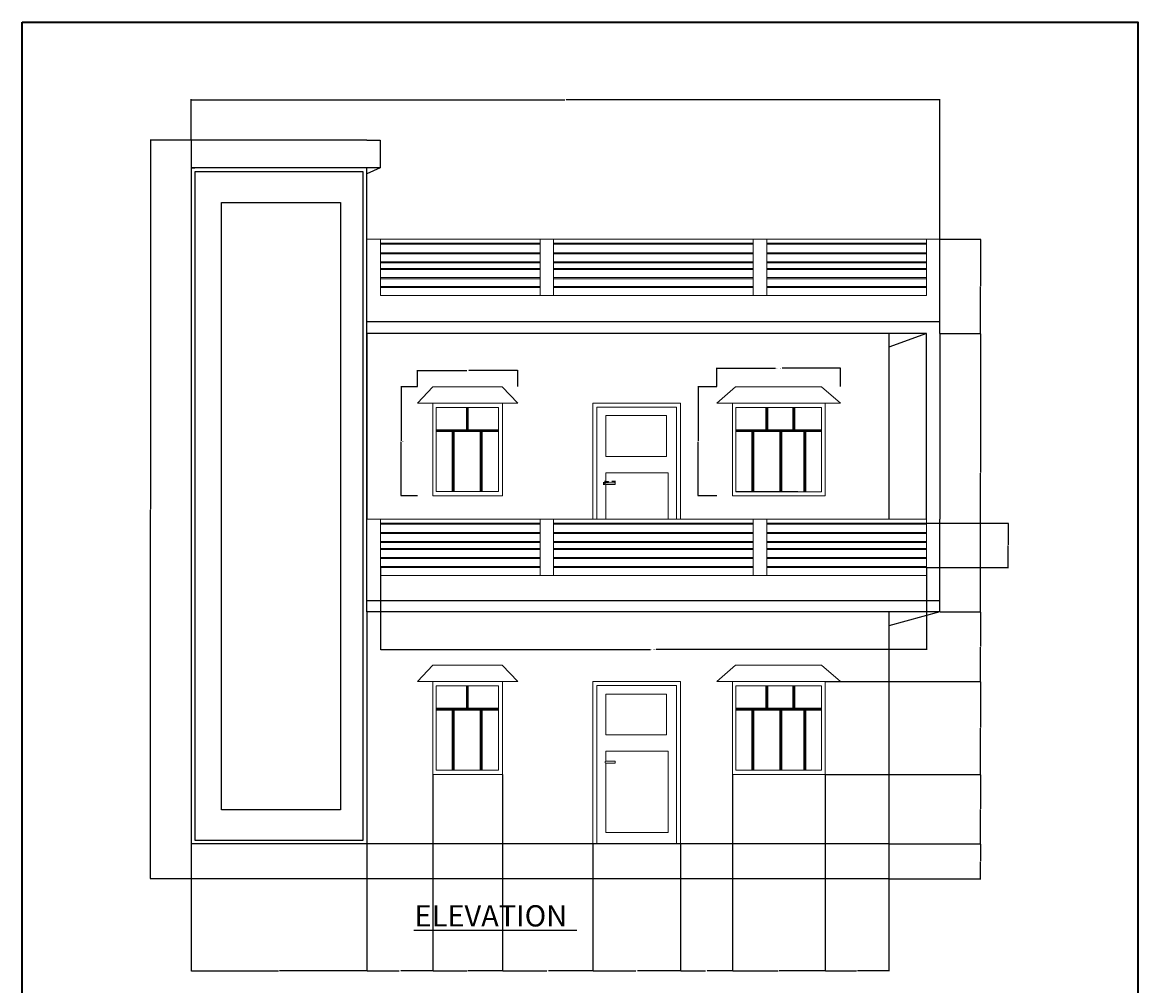
# Model space of a CAD drawing. Units: inches. Extents: x 1623 to 2200, y 2019 to 3010.
# Tile 6 of 6: x 1623 to 2200, y 2512 to 3010. Entities that reach past the tile are written whole.
import ezdxf

# ---------------------------------------------------------------- set-up
doc = ezdxf.new("R2010")
doc.units = ezdxf.units.IN
for name, color, linetype, lineweight in [('A-ANNO-DIMS', 2, 'Continuous', 18), ('A-ANNO-TITL', 7, 'Continuous', 25), ('A-ANNO-TTLB', 7, 'Continuous', 35), ('A-ELEV', 7, 'Continuous', 25), ('A-ELEV-DOOR', 3, 'Continuous', 18), ('A-ELEV-GLAZ', 4, 'Continuous', 18), ('A-ELEV-RAIL', 7, 'Continuous', 18)]:
    doc.layers.add(name, color=color, linetype=linetype, lineweight=lineweight)
doc.styles.get("Standard").update_dxf_attribs({"font": 'arial.ttf'})
doc.dimstyles.get("Standard").update_dxf_attribs({"dimtxt": 0.18, "dimasz": 0.18, "dimexe": 0.18, "dimexo": 0.0625, "dimgap": 0.09, "dimtad": 0, "dimtih": 1, "dimtoh": 1, "dimdec": 4, "dimzin": 0, "dimdsep": 46, "dimtxsty": 'Standard', "dimcen": 0.09, "dimadec": 0, "dimazin": 0, "dimtfac": 1, "dimtdec": 4, "dimtofl": 0, "dimtmove": 0, "dimatfit": 3, "dimfxl": 1, "dimtolj": 1, "dimtzin": 0, "dimarcsym": 0})

# ---------------------------------------------------------------- blocks, each defined once
blk = doc.blocks.new('WIN-HOODED-36-ELEV')
for p, q in [((0, 48), (8, 56.49)), ((8, 56.49), (43.77, 56.49)), ((52, 48), (43.77, 56.49)), ((8, 48), (0, 48)), ((8, 48), (8, 0)), ((44, 48), (8, 48)), ((44, 48), (44, 0)), ((44, 48), (52, 48)), ((25.79, 45.8), (25.29, 45.8)), ((25.29, 45.8), (25.29, 34.28)), ((25.79, 45.8), (25.79, 34.28)), ((26.29, 45.8), (25.79, 45.8)), ((26.29, 34.28), (26.29, 45.8)), ((9.7, 34.28), (41.87, 34.28)), ((9.7, 33.28), (9.7, 33.78)), ((9.7, 33.78), (41.87, 33.78)), ((41.87, 33.28), (9.7, 33.28)), ((18.52, 33.28), (18.02, 33.28)), ((18.02, 33.28), (18.02, 2.25)), ((18.52, 33.28), (18.52, 2.25)), ((19.02, 33.28), (18.52, 33.28)), ((19.02, 2.25), (19.02, 33.28)), ((25.79, 34.28), (26.29, 34.28)), ((32.47, 33.28), (32.47, 2.25)), ((32.97, 33.28), (32.97, 2.25)), ((33.47, 2.25), (33.47, 33.28)), ((41.87, 34.28), (41.87, 33.28)), ((44, 0), (8, 0)), ((18.52, 2.25), (19.02, 2.25))]:
    blk.add_line(p, q)
for points in [[(8, 48), (44, 48), (44, 0), (8, 0)], [(9.7, 45.8), (41.87, 45.8), (41.87, 2.25), (9.7, 2.25)]]:
    blk.add_lwpolyline(points, close=True)
blk = doc.blocks.new('WIN-HOODED-48-ELEV')
for p, q in [((0, 48), (9.64, 56.49)), ((9.64, 56.49), (54.05, 56.49)), ((64, 48), (54.05, 56.49)), ((8, 48), (0, 48)), ((56, 48), (8, 48)), ((8, 48), (8, 0)), ((56, 48), (56, 0)), ((56, 48), (64, 48)), ((25.38, 45.8), (25.38, 34.28)), ((25.88, 45.8), (25.88, 34.28)), ((26.38, 34.28), (26.38, 45.8)), ((39.3, 45.8), (39.3, 34.28)), ((39.8, 45.8), (39.8, 34.28)), ((40.3, 34.28), (40.3, 45.8)), ((9.79, 34.28), (54.04, 34.28)), ((9.79, 33.78), (54.04, 33.78)), ((54.04, 33.28), (9.79, 33.28)), ((18.61, 33.28), (18.11, 33.28)), ((18.11, 33.28), (18.11, 2.25)), ((18.61, 33.28), (18.61, 2.25)), ((19.11, 33.28), (18.61, 33.28)), ((19.11, 2.25), (19.11, 33.28)), ((25.88, 34.28), (26.38, 34.28)), ((32.57, 33.28), (32.57, 2.25)), ((33.07, 33.28), (33.07, 2.25)), ((33.57, 2.25), (33.57, 33.28)), ((45.02, 33.28), (45.02, 2.25)), ((45.52, 33.28), (45.52, 2.25)), ((46.02, 2.25), (46.02, 33.28)), ((56, 0), (8, 0))]:
    blk.add_line(p, q)
blk.add_lwpolyline([(41.96, 2.25), (9.79, 2.25), (9.79, 45.8), (41.96, 45.8)])
blk.add_lwpolyline([(9.79, 45.8), (54.04, 45.8), (54.04, 2.19), (9.79, 2.19)], close=True)
blk = doc.blocks.new('GUARD-INFILL-THREE-BAY')
for p, q in [((0, 22.98), (82.54, 22.98)), ((0, 22.44), (82.54, 22.44)), ((0, 18.02), (82.54, 18.02)), ((0, 17.48), (82.54, 17.48)), ((89.54, 22.98), (192.77, 22.98)), ((89.54, 22.44), (192.77, 22.44)), ((89.54, 18.02), (192.77, 18.02)), ((89.54, 17.48), (192.77, 17.48)), ((199.77, 22.98), (282.36, 22.98)), ((199.77, 22.44), (282.36, 22.44)), ((199.77, 18.02), (282.36, 18.02)), ((199.77, 17.48), (282.36, 17.48)), ((0, 13.4), (82.54, 13.4)), ((0, 12.86), (82.54, 12.86)), ((89.54, 13.4), (192.77, 13.4)), ((89.54, 12.86), (192.77, 12.86)), ((199.77, 13.4), (282.36, 13.4)), ((199.77, 12.86), (282.36, 12.86)), ((0, 9.89), (82.54, 9.89)), ((0, 9.34), (82.54, 9.34)), ((89.54, 9.89), (192.77, 9.89)), ((89.54, 9.34), (192.77, 9.34)), ((199.77, 9.89), (282.36, 9.89)), ((199.77, 9.34), (282.36, 9.34)), ((0, 5.16), (82.54, 5.16)), ((0, 4.62), (82.54, 4.62)), ((0, 0.54), (82.54, 0.54)), ((0, 0), (82.54, 0)), ((89.54, 5.16), (192.77, 5.16)), ((89.54, 4.62), (192.77, 4.62)), ((89.54, 0.54), (192.77, 0.54)), ((89.54, 0), (192.77, 0)), ((199.77, 5.16), (282.36, 5.16)), ((199.77, 4.62), (282.36, 4.62)), ((199.77, 0.54), (282.36, 0.54)), ((199.77, 0), (282.36, 0))]:
    blk.add_line(p, q)
blk = doc.blocks.new('DOOR-LEVER-ELEV')
blk.add_lwpolyline([(0.34, 0.92), (5.29, 0.92), (5.29, 0), (0.34, 0)])
blk.add_arc((0.48, 0.46), 0.478, 106.81153, 253.18847)
blk = doc.blocks.new('*D20')
at = {"layer": 'A-ANNO-DIMS', "color": 0, "lineweight": -2, "transparency": 16777216}
for p, q in [((1827.39, 2822.01), (1818.8, 2822.01)), ((1818.98, 2821.83), (1818.98, 2793.95)), ((1818.98, 2765.7), (1818.98, 2793.58)), ((1827.39, 2765.52), (1818.8, 2765.52))]:
    blk.add_line(p, q, dxfattribs=at)
at = {"layer": 'A-ANNO-DIMS', "color": 0, "transparency": 16777216}
for points in [[(1818.95, 2821.83), (1819.01, 2821.83), (1818.98, 2822.01)], [(1818.95, 2765.7), (1819.01, 2765.7), (1818.98, 2765.52)]]:
    blk.add_solid(points, dxfattribs=at)
at = {"layer": 'Defpoints', "color": 0, "transparency": 16777216}
for p in [(1818.98, 2822.01), (1827.45, 2822.01), (1827.45, 2765.52)]:
    blk.add_point(p, dxfattribs=at)
at = {"layer": 'A-ANNO-DIMS', "color": 0, "transparency": 16777216, "insert": (1818.98, 2793.77), "char_height": 0.18, "attachment_point": 5}
blk.add_mtext('\\A1;HOODED WINDOW 56 TYP.', dxfattribs=at)
blk = doc.blocks.new('*D21')
at = {"layer": 'A-ANNO-DIMS', "color": 0, "lineweight": -2, "transparency": 16777216}
for p, q in [((1827.45, 2822.07), (1827.45, 2830.66)), ((1827.63, 2830.48), (1852.93, 2830.48)), ((1879.27, 2830.48), (1853.98, 2830.48)), ((1879.45, 2822.07), (1879.45, 2830.66))]:
    blk.add_line(p, q, dxfattribs=at)
at = {"layer": 'A-ANNO-DIMS', "color": 0, "transparency": 16777216}
for points in [[(1827.63, 2830.51), (1827.63, 2830.45), (1827.45, 2830.48)], [(1879.27, 2830.51), (1879.27, 2830.45), (1879.45, 2830.48)]]:
    blk.add_solid(points, dxfattribs=at)
at = {"layer": 'Defpoints', "color": 0, "transparency": 16777216}
for p in [(1879.45, 2830.48), (1827.45, 2822.01), (1879.45, 2822.01)]:
    blk.add_point(p, dxfattribs=at)
at = {"layer": 'A-ANNO-DIMS', "color": 0, "transparency": 16777216, "insert": (1853.45, 2830.48), "char_height": 0.18, "attachment_point": 5}
blk.add_mtext('\\A1;52 TYP.', dxfattribs=at)
blk = doc.blocks.new('*D22')
at = {"layer": 'A-ANNO-DIMS', "color": 0, "lineweight": -2, "transparency": 16777216}
for p, q in [((1982.33, 2822.07), (1982.33, 2831.79)), ((1982.51, 2831.61), (2012.63, 2831.61)), ((2046.15, 2831.61), (2016.02, 2831.61)), ((2046.33, 2822.07), (2046.33, 2831.79))]:
    blk.add_line(p, q, dxfattribs=at)
at = {"layer": 'A-ANNO-DIMS', "color": 0, "transparency": 16777216}
for points in [[(1982.51, 2831.64), (1982.51, 2831.58), (1982.33, 2831.61)], [(2046.15, 2831.64), (2046.15, 2831.58), (2046.33, 2831.61)]]:
    blk.add_solid(points, dxfattribs=at)
at = {"layer": 'Defpoints', "color": 0, "transparency": 16777216}
for p in [(2046.33, 2831.61), (1982.33, 2822.01), (2046.33, 2822.01)]:
    blk.add_point(p, dxfattribs=at)
at = {"layer": 'A-ANNO-DIMS', "color": 0, "transparency": 16777216, "insert": (2014.33, 2831.61), "char_height": 0.18, "attachment_point": 5}
blk.add_mtext('\\A1;HOODED WINDOW 64 TYP.', dxfattribs=at)
blk = doc.blocks.new('*D23')
at = {"layer": 'A-ANNO-DIMS', "color": 0, "lineweight": -2, "transparency": 16777216}
for p, q in [((1982.26, 2822.01), (1972.55, 2822.01)), ((1972.73, 2821.83), (1972.73, 2793.95)), ((1972.73, 2765.7), (1972.73, 2793.58)), ((1982.26, 2765.52), (1972.55, 2765.52))]:
    blk.add_line(p, q, dxfattribs=at)
at = {"layer": 'A-ANNO-DIMS', "color": 0, "transparency": 16777216}
for points in [[(1972.7, 2821.83), (1972.76, 2821.83), (1972.73, 2822.01)], [(1972.7, 2765.7), (1972.76, 2765.7), (1972.73, 2765.52)]]:
    blk.add_solid(points, dxfattribs=at)
at = {"layer": 'Defpoints', "color": 0, "transparency": 16777216}
for p in [(1972.73, 2822.01), (1982.33, 2822.01), (1982.33, 2765.52)]:
    blk.add_point(p, dxfattribs=at)
at = {"layer": 'A-ANNO-DIMS', "color": 0, "transparency": 16777216, "insert": (1972.73, 2793.77), "char_height": 0.18, "attachment_point": 5}
blk.add_mtext('\\A1;56 TYP.', dxfattribs=at)
blk = doc.blocks.new('*D24')
at = {"layer": 'A-ANNO-DIMS', "color": 0, "lineweight": -2, "transparency": 16777216}
for p, q in [((1808.33, 2728.48), (1808.33, 2686.01)), ((2090.69, 2728.48), (2090.69, 2686.01)), ((1808.51, 2686.19), (1948.01, 2686.19)), ((2090.51, 2686.19), (1951, 2686.19))]:
    blk.add_line(p, q, dxfattribs=at)
at = {"layer": 'A-ANNO-DIMS', "color": 0, "transparency": 16777216}
for points in [[(1808.51, 2686.22), (1808.51, 2686.16), (1808.33, 2686.19)], [(2090.51, 2686.22), (2090.51, 2686.16), (2090.69, 2686.19)]]:
    blk.add_solid(points, dxfattribs=at)
at = {"layer": 'Defpoints', "color": 0, "transparency": 16777216}
for p in [(1808.33, 2728.54), (2090.69, 2728.54), (2090.69, 2686.19)]:
    blk.add_point(p, dxfattribs=at)
at = {"layer": 'A-ANNO-DIMS', "color": 0, "transparency": 16777216, "insert": (1949.51, 2686.19), "char_height": 0.18, "attachment_point": 5}
blk.add_mtext('\\A1;GUARD INFILL 282 TYP.', dxfattribs=at)
blk = doc.blocks.new('*D25')
at = {"layer": 'A-ANNO-DIMS', "color": 0, "lineweight": -2, "transparency": 16777216}
for p, q in [((2090.75, 2751.52), (2133.22, 2751.52)), ((2133.04, 2751.34), (2133.04, 2740.21)), ((2133.04, 2728.72), (2133.04, 2739.85)), ((2090.75, 2728.54), (2133.22, 2728.54))]:
    blk.add_line(p, q, dxfattribs=at)
at = {"layer": 'A-ANNO-DIMS', "color": 0, "transparency": 16777216}
for points in [[(2133.01, 2751.34), (2133.07, 2751.34), (2133.04, 2751.52)], [(2133.01, 2728.72), (2133.07, 2728.72), (2133.04, 2728.54)]]:
    blk.add_solid(points, dxfattribs=at)
at = {"layer": 'Defpoints', "color": 0, "transparency": 16777216}
for p in [(2090.69, 2751.52), (2133.04, 2751.52), (2090.69, 2728.54)]:
    blk.add_point(p, dxfattribs=at)
at = {"layer": 'A-ANNO-DIMS', "color": 0, "transparency": 16777216, "insert": (2133.04, 2740.03), "char_height": 0.18, "attachment_point": 5}
blk.add_mtext('\\A1;23 TYP.', dxfattribs=at)
blk = doc.blocks.new('*D26')
at = {"layer": 'A-ANNO-DIMS', "color": 0, "lineweight": -2, "transparency": 16777216}
for p, q in [((1924.49, 2772.35), (1924.49, 2773.26)), ((1924.67, 2773.08), (1926.24, 2773.08)), ((1929.6, 2773.08), (1928.04, 2773.08)), ((1929.78, 2772.35), (1929.78, 2773.26))]:
    blk.add_line(p, q, dxfattribs=at)
at = {"layer": 'A-ANNO-DIMS', "color": 0, "transparency": 16777216}
for points in [[(1924.67, 2773.11), (1924.67, 2773.05), (1924.49, 2773.08)], [(1929.6, 2773.11), (1929.6, 2773.05), (1929.78, 2773.08)]]:
    blk.add_solid(points, dxfattribs=at)
at = {"layer": 'Defpoints', "color": 0, "transparency": 16777216}
for p in [(1924.49, 2772.28), (1929.78, 2773.08), (1929.78, 2772.28)]:
    blk.add_point(p, dxfattribs=at)
at = {"layer": 'A-ANNO-DIMS', "color": 0, "transparency": 16777216, "insert": (1927.14, 2773.08), "char_height": 0.18, "attachment_point": 5}
blk.add_mtext('\\A1;LEVER 5 TYP.', dxfattribs=at)
blk = doc.blocks.new('*D27')
at = {"layer": 'A-ANNO-DIMS', "color": 0, "lineweight": -2, "transparency": 16777216}
for p, q in [((1924.43, 2772.28), (1923.52, 2772.28)), ((1924.43, 2771.37), (1923.52, 2771.37)), ((1923.7, 2772.1), (1923.7, 2772.01)), ((1923.7, 2771.55), (1923.7, 2771.65))]:
    blk.add_line(p, q, dxfattribs=at)
at = {"layer": 'A-ANNO-DIMS', "color": 0, "transparency": 16777216}
for points in [[(1923.67, 2772.1), (1923.73, 2772.1), (1923.7, 2772.28)], [(1923.67, 2771.55), (1923.73, 2771.55), (1923.7, 2771.37)]]:
    blk.add_solid(points, dxfattribs=at)
at = {"layer": 'Defpoints', "color": 0, "transparency": 16777216}
for p in [(1923.7, 2772.28), (1924.49, 2772.28), (1924.49, 2771.37)]:
    blk.add_point(p, dxfattribs=at)
at = {"layer": 'A-ANNO-DIMS', "color": 0, "transparency": 16777216, "insert": (1923.7, 2771.83), "char_height": 0.18, "attachment_point": 5}
blk.add_mtext('\\A1;1 TYP.', dxfattribs=at)
blk = doc.blocks.new('*D44')
at = {"layer": 'A-ANNO-DIMS', "color": 0, "lineweight": -2, "transparency": 16777216}
for p, q in [((1710.33, 2949.6), (1710.33, 2970.66)), ((1710.51, 2970.48), (1903.61, 2970.48)), ((2097.51, 2970.48), (1904.4, 2970.48)), ((2097.69, 2898.32), (2097.69, 2970.66))]:
    blk.add_line(p, q, dxfattribs=at)
at = {"layer": 'A-ANNO-DIMS', "color": 0, "transparency": 16777216}
for points in [[(1710.51, 2970.51), (1710.51, 2970.45), (1710.33, 2970.48)], [(2097.51, 2970.51), (2097.51, 2970.45), (2097.69, 2970.48)]]:
    blk.add_solid(points, dxfattribs=at)
at = {"layer": 'Defpoints', "color": 0, "transparency": 16777216}
for p in [(2097.69, 2970.48), (1710.33, 2949.53), (2097.69, 2898.26)]:
    blk.add_point(p, dxfattribs=at)
at = {"layer": 'A-ANNO-DIMS', "color": 0, "transparency": 16777216, "insert": (1904.01, 2970.48), "char_height": 0.18, "attachment_point": 5}
blk.add_mtext('\\A1;387.4', dxfattribs=at)
blk = doc.blocks.new('*D45')
at = {"layer": 'A-ANNO-DIMS', "color": 0, "lineweight": -2, "transparency": 16777216}
for p, q in [((1710.26, 2949.53), (1689.2, 2949.53)), ((1689.38, 2949.35), (1689.38, 2758.71)), ((1689.38, 2567.7), (1689.38, 2758.34)), ((1710.26, 2567.52), (1689.2, 2567.52))]:
    blk.add_line(p, q, dxfattribs=at)
at = {"layer": 'A-ANNO-DIMS', "color": 0, "transparency": 16777216}
for points in [[(1689.35, 2949.35), (1689.41, 2949.35), (1689.38, 2949.53)], [(1689.35, 2567.7), (1689.41, 2567.7), (1689.38, 2567.52)]]:
    blk.add_solid(points, dxfattribs=at)
at = {"layer": 'Defpoints', "color": 0, "transparency": 16777216}
for p in [(1689.38, 2949.53), (1710.33, 2949.53), (1710.33, 2567.52)]:
    blk.add_point(p, dxfattribs=at)
at = {"layer": 'A-ANNO-DIMS', "color": 0, "transparency": 16777216, "insert": (1689.38, 2758.53), "char_height": 0.18, "attachment_point": 5}
blk.add_mtext('\\A1;382', dxfattribs=at)
blk = doc.blocks.new('*D46')
at = {"layer": 'A-ANNO-DIMS', "color": 0, "lineweight": -2, "transparency": 16777216}
for p, q in [((2071.39, 2585.52), (2118.82, 2585.52)), ((2118.64, 2585.34), (2118.64, 2576.7)), ((2118.64, 2567.7), (2118.64, 2576.34)), ((2071.39, 2567.52), (2118.82, 2567.52))]:
    blk.add_line(p, q, dxfattribs=at)
at = {"layer": 'A-ANNO-DIMS', "color": 0, "transparency": 16777216}
for points in [[(2118.61, 2585.34), (2118.67, 2585.34), (2118.64, 2585.52)], [(2118.61, 2567.7), (2118.67, 2567.7), (2118.64, 2567.52)]]:
    blk.add_solid(points, dxfattribs=at)
at = {"layer": 'Defpoints', "color": 0, "transparency": 16777216}
for p in [(2071.33, 2585.52), (2118.64, 2585.52), (2071.33, 2567.52)]:
    blk.add_point(p, dxfattribs=at)
at = {"layer": 'A-ANNO-DIMS', "color": 0, "transparency": 16777216, "insert": (2118.64, 2576.52), "char_height": 0.18, "attachment_point": 5}
blk.add_mtext('\\A1;18', dxfattribs=at)
blk = doc.blocks.new('*D47')
at = {"layer": 'A-ANNO-DIMS', "color": 0, "lineweight": -2, "transparency": 16777216}
for p, q in [((2038.39, 2621.52), (2118.82, 2621.52)), ((2118.64, 2621.34), (2118.64, 2603.7)), ((2118.64, 2585.7), (2118.64, 2603.34)), ((2071.39, 2585.52), (2118.82, 2585.52))]:
    blk.add_line(p, q, dxfattribs=at)
at = {"layer": 'A-ANNO-DIMS', "color": 0, "transparency": 16777216}
for points in [[(2118.61, 2621.34), (2118.67, 2621.34), (2118.64, 2621.52)], [(2118.61, 2585.7), (2118.67, 2585.7), (2118.64, 2585.52)]]:
    blk.add_solid(points, dxfattribs=at)
at = {"layer": 'Defpoints', "color": 0, "transparency": 16777216}
for p in [(2038.33, 2621.52), (2118.64, 2621.52), (2071.33, 2585.52)]:
    blk.add_point(p, dxfattribs=at)
at = {"layer": 'A-ANNO-DIMS', "color": 0, "transparency": 16777216, "insert": (2118.64, 2603.52), "char_height": 0.18, "attachment_point": 5}
blk.add_mtext('\\A1;36', dxfattribs=at)
blk = doc.blocks.new('*D48')
at = {"layer": 'A-ANNO-DIMS', "color": 0, "lineweight": -2, "transparency": 16777216}
for p, q in [((2038.39, 2669.52), (2118.82, 2669.52)), ((2118.64, 2669.34), (2118.64, 2645.7)), ((2118.64, 2621.7), (2118.64, 2645.34)), ((2038.39, 2621.52), (2118.82, 2621.52))]:
    blk.add_line(p, q, dxfattribs=at)
at = {"layer": 'A-ANNO-DIMS', "color": 0, "transparency": 16777216}
for points in [[(2118.61, 2669.34), (2118.67, 2669.34), (2118.64, 2669.52)], [(2118.61, 2621.7), (2118.67, 2621.7), (2118.64, 2621.52)]]:
    blk.add_solid(points, dxfattribs=at)
at = {"layer": 'Defpoints', "color": 0, "transparency": 16777216}
for p in [(2038.33, 2669.52), (2118.64, 2669.52), (2038.33, 2621.52)]:
    blk.add_point(p, dxfattribs=at)
at = {"layer": 'A-ANNO-DIMS', "color": 0, "transparency": 16777216, "insert": (2118.64, 2645.52), "char_height": 0.18, "attachment_point": 5}
blk.add_mtext('\\A1;48', dxfattribs=at)
blk = doc.blocks.new('*D49')
at = {"layer": 'A-ANNO-DIMS', "color": 0, "lineweight": -2, "transparency": 16777216}
for p, q in [((2097.75, 2705.52), (2118.82, 2705.52)), ((2118.64, 2705.34), (2118.64, 2687.7)), ((2118.64, 2669.7), (2118.64, 2687.34)), ((2038.39, 2669.52), (2118.82, 2669.52))]:
    blk.add_line(p, q, dxfattribs=at)
at = {"layer": 'A-ANNO-DIMS', "color": 0, "transparency": 16777216}
for points in [[(2118.61, 2705.34), (2118.67, 2705.34), (2118.64, 2705.52)], [(2118.61, 2669.7), (2118.67, 2669.7), (2118.64, 2669.52)]]:
    blk.add_solid(points, dxfattribs=at)
at = {"layer": 'Defpoints', "color": 0, "transparency": 16777216}
for p in [(2097.69, 2705.52), (2118.64, 2705.52), (2038.33, 2669.52)]:
    blk.add_point(p, dxfattribs=at)
at = {"layer": 'A-ANNO-DIMS', "color": 0, "transparency": 16777216, "insert": (2118.64, 2687.52), "char_height": 0.18, "attachment_point": 5}
blk.add_mtext('\\A1;36', dxfattribs=at)
blk = doc.blocks.new('*D50')
at = {"layer": 'A-ANNO-DIMS', "color": 0, "lineweight": -2, "transparency": 16777216}
for p, q in [((2097.75, 2849.52), (2118.82, 2849.52)), ((2118.64, 2849.34), (2118.64, 2777.7)), ((2118.64, 2705.7), (2118.64, 2777.34)), ((2097.75, 2705.52), (2118.82, 2705.52))]:
    blk.add_line(p, q, dxfattribs=at)
at = {"layer": 'A-ANNO-DIMS', "color": 0, "transparency": 16777216}
for points in [[(2118.61, 2849.34), (2118.67, 2849.34), (2118.64, 2849.52)], [(2118.61, 2705.7), (2118.67, 2705.7), (2118.64, 2705.52)]]:
    blk.add_solid(points, dxfattribs=at)
at = {"layer": 'Defpoints', "color": 0, "transparency": 16777216}
for p in [(2097.69, 2849.52), (2118.64, 2849.52), (2097.69, 2705.52)]:
    blk.add_point(p, dxfattribs=at)
at = {"layer": 'A-ANNO-DIMS', "color": 0, "transparency": 16777216, "insert": (2118.64, 2777.52), "char_height": 0.18, "attachment_point": 5}
blk.add_mtext('\\A1;144', dxfattribs=at)
blk = doc.blocks.new('*D51')
at = {"layer": 'A-ANNO-DIMS', "color": 0, "lineweight": -2, "transparency": 16777216}
for p, q in [((2097.75, 2898.26), (2118.82, 2898.26)), ((2118.64, 2898.08), (2118.64, 2874.07)), ((2118.64, 2849.7), (2118.64, 2873.71)), ((2097.75, 2849.52), (2118.82, 2849.52))]:
    blk.add_line(p, q, dxfattribs=at)
at = {"layer": 'A-ANNO-DIMS', "color": 0, "transparency": 16777216}
for points in [[(2118.61, 2898.08), (2118.67, 2898.08), (2118.64, 2898.26)], [(2118.61, 2849.7), (2118.67, 2849.7), (2118.64, 2849.52)]]:
    blk.add_solid(points, dxfattribs=at)
at = {"layer": 'Defpoints', "color": 0, "transparency": 16777216}
for p in [(2097.69, 2898.26), (2118.64, 2898.26), (2097.69, 2849.52)]:
    blk.add_point(p, dxfattribs=at)
at = {"layer": 'A-ANNO-DIMS', "color": 0, "transparency": 16777216, "insert": (2118.64, 2873.89), "char_height": 0.18, "attachment_point": 5}
blk.add_mtext('\\A1;48.74', dxfattribs=at)
blk = doc.blocks.new('*D52')
at = {"layer": 'A-ANNO-DIMS', "color": 0, "lineweight": -2, "transparency": 16777216}
for p, q in [((1801.33, 2585.46), (1801.33, 2519.8)), ((1710.33, 2567.46), (1710.33, 2519.8)), ((1710.51, 2519.98), (1755.62, 2519.98)), ((1801.15, 2519.98), (1756.03, 2519.98))]:
    blk.add_line(p, q, dxfattribs=at)
at = {"layer": 'A-ANNO-DIMS', "color": 0, "transparency": 16777216}
for points in [[(1710.51, 2520.01), (1710.51, 2519.95), (1710.33, 2519.98)], [(1801.15, 2520.01), (1801.15, 2519.95), (1801.33, 2519.98)]]:
    blk.add_solid(points, dxfattribs=at)
at = {"layer": 'Defpoints', "color": 0, "transparency": 16777216}
for p in [(1801.33, 2585.52), (1710.33, 2567.52), (1801.33, 2519.98)]:
    blk.add_point(p, dxfattribs=at)
at = {"layer": 'A-ANNO-DIMS', "color": 0, "transparency": 16777216, "insert": (1755.83, 2519.98), "char_height": 0.18, "attachment_point": 5}
blk.add_mtext('\\A1;91', dxfattribs=at)
blk = doc.blocks.new('*D53')
at = {"layer": 'A-ANNO-DIMS', "color": 0, "lineweight": -2, "transparency": 16777216}
for p, q in [((1835.45, 2621.46), (1835.45, 2519.8)), ((1801.33, 2585.46), (1801.33, 2519.8)), ((1801.51, 2519.98), (1818, 2519.98)), ((1835.27, 2519.98), (1818.78, 2519.98))]:
    blk.add_line(p, q, dxfattribs=at)
at = {"layer": 'A-ANNO-DIMS', "color": 0, "transparency": 16777216}
for points in [[(1801.51, 2520.01), (1801.51, 2519.95), (1801.33, 2519.98)], [(1835.27, 2520.01), (1835.27, 2519.95), (1835.45, 2519.98)]]:
    blk.add_solid(points, dxfattribs=at)
at = {"layer": 'Defpoints', "color": 0, "transparency": 16777216}
for p in [(1835.45, 2621.52), (1801.33, 2585.52), (1835.45, 2519.98)]:
    blk.add_point(p, dxfattribs=at)
at = {"layer": 'A-ANNO-DIMS', "color": 0, "transparency": 16777216, "insert": (1818.39, 2519.98), "char_height": 0.18, "attachment_point": 5}
blk.add_mtext('\\A1;34.13', dxfattribs=at)
blk = doc.blocks.new('*D54')
at = {"layer": 'A-ANNO-DIMS', "color": 0, "lineweight": -2, "transparency": 16777216}
for p, q in [((1835.45, 2621.46), (1835.45, 2519.8)), ((1871.45, 2621.46), (1871.45, 2519.8)), ((1835.63, 2519.98), (1853.24, 2519.98)), ((1871.27, 2519.98), (1853.67, 2519.98))]:
    blk.add_line(p, q, dxfattribs=at)
at = {"layer": 'A-ANNO-DIMS', "color": 0, "transparency": 16777216}
for points in [[(1835.63, 2520.01), (1835.63, 2519.95), (1835.45, 2519.98)], [(1871.27, 2520.01), (1871.27, 2519.95), (1871.45, 2519.98)]]:
    blk.add_solid(points, dxfattribs=at)
at = {"layer": 'Defpoints', "color": 0, "transparency": 16777216}
for p in [(1835.45, 2621.52), (1871.45, 2621.52), (1871.45, 2519.98)]:
    blk.add_point(p, dxfattribs=at)
at = {"layer": 'A-ANNO-DIMS', "color": 0, "transparency": 16777216, "insert": (1853.45, 2519.98), "char_height": 0.18, "attachment_point": 5}
blk.add_mtext('\\A1;36', dxfattribs=at)
blk = doc.blocks.new('*D55')
at = {"layer": 'A-ANNO-DIMS', "color": 0, "lineweight": -2, "transparency": 16777216}
for p, q in [((1871.45, 2621.46), (1871.45, 2519.8)), ((1918.23, 2585.46), (1918.23, 2519.8)), ((1871.63, 2519.98), (1894.44, 2519.98)), ((1918.05, 2519.98), (1895.24, 2519.98))]:
    blk.add_line(p, q, dxfattribs=at)
at = {"layer": 'A-ANNO-DIMS', "color": 0, "transparency": 16777216}
for points in [[(1871.63, 2520.01), (1871.63, 2519.95), (1871.45, 2519.98)], [(1918.05, 2520.01), (1918.05, 2519.95), (1918.23, 2519.98)]]:
    blk.add_solid(points, dxfattribs=at)
at = {"layer": 'Defpoints', "color": 0, "transparency": 16777216}
for p in [(1871.45, 2621.52), (1918.23, 2585.52), (1918.23, 2519.98)]:
    blk.add_point(p, dxfattribs=at)
at = {"layer": 'A-ANNO-DIMS', "color": 0, "transparency": 16777216, "insert": (1894.84, 2519.98), "char_height": 0.18, "attachment_point": 5}
blk.add_mtext('\\A1;46.77', dxfattribs=at)
blk = doc.blocks.new('*D56')
at = {"layer": 'A-ANNO-DIMS', "color": 0, "lineweight": -2, "transparency": 16777216}
for p, q in [((1918.23, 2585.46), (1918.23, 2519.8)), ((1963.44, 2585.46), (1963.44, 2519.8)), ((1918.41, 2519.98), (1940.45, 2519.98)), ((1963.26, 2519.98), (1941.21, 2519.98))]:
    blk.add_line(p, q, dxfattribs=at)
at = {"layer": 'A-ANNO-DIMS', "color": 0, "transparency": 16777216}
for points in [[(1918.41, 2520.01), (1918.41, 2519.95), (1918.23, 2519.98)], [(1963.26, 2520.01), (1963.26, 2519.95), (1963.44, 2519.98)]]:
    blk.add_solid(points, dxfattribs=at)
at = {"layer": 'Defpoints', "color": 0, "transparency": 16777216}
for p in [(1918.23, 2585.52), (1963.44, 2585.52), (1963.44, 2519.98)]:
    blk.add_point(p, dxfattribs=at)
at = {"layer": 'A-ANNO-DIMS', "color": 0, "transparency": 16777216, "insert": (1940.83, 2519.98), "char_height": 0.18, "attachment_point": 5}
blk.add_mtext('\\A1;45.21', dxfattribs=at)
blk = doc.blocks.new('*D57')
at = {"layer": 'A-ANNO-DIMS', "color": 0, "lineweight": -2, "transparency": 16777216}
for p, q in [((1990.33, 2621.46), (1990.33, 2519.8)), ((1963.44, 2585.46), (1963.44, 2519.8)), ((1963.62, 2519.98), (1976.42, 2519.98)), ((1990.15, 2519.98), (1977.35, 2519.98))]:
    blk.add_line(p, q, dxfattribs=at)
at = {"layer": 'A-ANNO-DIMS', "color": 0, "transparency": 16777216}
for points in [[(1963.62, 2520.01), (1963.62, 2519.95), (1963.44, 2519.98)], [(1990.15, 2520.01), (1990.15, 2519.95), (1990.33, 2519.98)]]:
    blk.add_solid(points, dxfattribs=at)
at = {"layer": 'Defpoints', "color": 0, "transparency": 16777216}
for p in [(1990.33, 2621.52), (1963.44, 2585.52), (1990.33, 2519.98)]:
    blk.add_point(p, dxfattribs=at)
at = {"layer": 'A-ANNO-DIMS', "color": 0, "transparency": 16777216, "insert": (1976.88, 2519.98), "char_height": 0.18, "attachment_point": 5}
blk.add_mtext('\\A1;26.886', dxfattribs=at)
blk = doc.blocks.new('*D58')
at = {"layer": 'A-ANNO-DIMS', "color": 0, "lineweight": -2, "transparency": 16777216}
for p, q in [((1990.33, 2621.46), (1990.33, 2519.8)), ((2038.33, 2621.46), (2038.33, 2519.8)), ((1990.51, 2519.98), (2014.1, 2519.98)), ((2038.15, 2519.98), (2014.55, 2519.98))]:
    blk.add_line(p, q, dxfattribs=at)
at = {"layer": 'A-ANNO-DIMS', "color": 0, "transparency": 16777216}
for points in [[(1990.51, 2520.01), (1990.51, 2519.95), (1990.33, 2519.98)], [(2038.15, 2520.01), (2038.15, 2519.95), (2038.33, 2519.98)]]:
    blk.add_solid(points, dxfattribs=at)
at = {"layer": 'Defpoints', "color": 0, "transparency": 16777216}
for p in [(1990.33, 2621.52), (2038.33, 2621.52), (2038.33, 2519.98)]:
    blk.add_point(p, dxfattribs=at)
at = {"layer": 'A-ANNO-DIMS', "color": 0, "transparency": 16777216, "insert": (2014.33, 2519.98), "char_height": 0.18, "attachment_point": 5}
blk.add_mtext('\\A1;48', dxfattribs=at)
blk = doc.blocks.new('*D59')
at = {"layer": 'A-ANNO-DIMS', "color": 0, "lineweight": -2, "transparency": 16777216}
for p, q in [((2038.33, 2621.46), (2038.33, 2519.8)), ((2071.33, 2567.46), (2071.33, 2519.8)), ((2038.51, 2519.98), (2054.61, 2519.98)), ((2071.15, 2519.98), (2055.04, 2519.98))]:
    blk.add_line(p, q, dxfattribs=at)
at = {"layer": 'A-ANNO-DIMS', "color": 0, "transparency": 16777216}
for points in [[(2038.51, 2520.01), (2038.51, 2519.95), (2038.33, 2519.98)], [(2071.15, 2520.01), (2071.15, 2519.95), (2071.33, 2519.98)]]:
    blk.add_solid(points, dxfattribs=at)
at = {"layer": 'Defpoints', "color": 0, "transparency": 16777216}
for p in [(2038.33, 2621.52), (2071.33, 2567.52), (2071.33, 2519.98)]:
    blk.add_point(p, dxfattribs=at)
at = {"layer": 'A-ANNO-DIMS', "color": 0, "transparency": 16777216, "insert": (2054.83, 2519.98), "char_height": 0.18, "attachment_point": 5}
blk.add_mtext('\\A1;33', dxfattribs=at)

msp = doc.modelspace()

# ---------------------------------------------------------------- linework, layer by layer
at = {"layer": 'A-ANNO-TITL'}
for p, q in [((1825.6086, 2540.9271), (1893.05, 2540.9271)), ((1893.05, 2540.9271), (1909.8099, 2540.9271))]:
    msp.add_line(p, q, dxfattribs=at)
at = {"layer": 'A-ANNO-TTLB'}
msp.add_lwpolyline([(1623.0453, 3010.4913), (2200.0052, 3010.4913), (2200.0052, 2019.4245), (1623.0453, 2019.4245)], close=True, dxfattribs=at)
at = {"layer": 'A-ELEV'}
for p, q in [((1801.3258, 2949.5338), (1710.3258, 2949.5338)), ((1710.3258, 2949.5338), (1710.3258, 2897.5191)), ((1801.3258, 2949.5338), (1808.1651, 2949.5338)), ((1808.1651, 2949.5338), (1808.1651, 2935.1751)), ((1801.3258, 2935.1751), (1710.3258, 2935.1751)), ((1710.3258, 2935.1751), (1712.3258, 2935.1751)), ((1712.3258, 2933.1751), (1712.3258, 2587.5191)), ((1799.3258, 2933.1751), (1712.3258, 2933.1751)), ((1799.3258, 2587.5191), (1799.3258, 2933.1751)), ((1801.3258, 2705.5191), (1801.3258, 2935.1751)), ((1808.1651, 2935.1751), (1801.3258, 2935.1751)), ((1808.1651, 2935.1751), (1801.3258, 2932.087)), ((1710.3258, 2897.5191), (1710.3258, 2711.5191)), ((2097.6881, 2849.5191), (2097.6881, 2898.2603)), ((2097.6881, 2855.5191), (1801.3258, 2855.5191)), ((2090.6881, 2849.5191), (1801.3258, 2849.5191)), ((1801.3258, 2849.5191), (1801.3258, 2753.5191)), ((2071.3258, 2849.5191), (2071.3258, 2753.5191)), ((2090.6881, 2849.5191), (2071.3258, 2842.4338)), ((2090.6881, 2753.5191), (2090.6881, 2849.5191)), ((2097.6881, 2849.5191), (2097.6881, 2753.5191)), ((1710.3258, 2753.5191), (1710.3258, 2567.5191)), ((2097.6881, 2705.5191), (2097.6881, 2753.5191)), ((1801.3258, 2709.5191), (1801.3258, 2711.5191)), ((1801.3258, 2711.5191), (2097.6881, 2711.5191)), ((1801.3258, 2707.5191), (1801.3258, 2709.5191)), ((1801.3258, 2705.5191), (1801.3258, 2707.5191)), ((2097.6881, 2705.5191), (1801.3258, 2705.5191)), ((1801.3258, 2705.5191), (1801.3258, 2585.5191)), ((2071.3258, 2705.5191), (2071.3258, 2567.5191)), ((2097.6881, 2705.5191), (2071.3258, 2698.3424)), ((2071.3258, 2585.5191), (1710.3258, 2585.5191)), ((1712.3258, 2587.5191), (1799.3258, 2587.5191)), ((2071.3258, 2567.5191), (1710.3258, 2567.5191))]:
    msp.add_line(p, q, dxfattribs=at)
msp.add_lwpolyline([(1726.1356, 2917.3294), (1787.7104, 2917.3294), (1787.7104, 2603.2285), (1726.1356, 2603.2285)], close=True, dxfattribs=at)
at = {"layer": 'A-ELEV-DOOR'}
for p, q in [((1963.4402, 2813.5191), (1918.2273, 2813.5191)), ((1918.2273, 2813.5191), (1918.2273, 2753.5191)), ((1963.4402, 2813.5191), (1918.2273, 2813.5191)), ((1918.2273, 2813.5191), (1918.2273, 2753.5191)), ((1920.2273, 2753.5191), (1920.2273, 2811.5191)), ((1920.2273, 2811.5191), (1961.4402, 2811.5191)), ((1961.4402, 2811.5191), (1961.4402, 2753.5191)), ((1963.4402, 2813.5191), (1963.4402, 2753.5191)), ((1963.4402, 2813.5191), (1963.4402, 2753.5191)), ((1918.2273, 2669.5191), (1918.2273, 2585.5191)), ((1963.4402, 2669.5191), (1918.2273, 2669.5191)), ((1920.2273, 2585.5191), (1920.2273, 2667.5191)), ((1920.2273, 2667.5191), (1961.4402, 2667.5191)), ((1961.4402, 2667.5191), (1961.4402, 2585.5191)), ((1963.4402, 2669.5191), (1963.4402, 2585.5191)), ((1918.2273, 2585.5191), (1920.2273, 2585.5191))]:
    msp.add_line(p, q, dxfattribs=at)
for points in [[(1918.2273, 2753.5191), (1918.2273, 2813.5191), (1963.4402, 2813.5191), (1963.4402, 2753.5191)], [(1918.2273, 2753.5191), (1918.2273, 2813.5191), (1963.4402, 2813.5191), (1963.4402, 2753.5191)], [(1924.8346, 2772.2848), (1924.8346, 2777.5634), (1957.072, 2777.5634), (1957.072, 2753.5191)], [(1924.8346, 2753.5191), (1924.8346, 2771.3692)], [(1924.8346, 2628.2848), (1924.8346, 2633.5634), (1957.072, 2633.5634), (1957.072, 2591.4369), (1924.8346, 2591.4369), (1924.8346, 2627.3692)]]:
    msp.add_lwpolyline(points, dxfattribs=at)
for points in [[(1924.8346, 2807.052), (1956.337, 2807.052), (1956.337, 2786.0108), (1924.8346, 2786.0108)], [(1918.2273, 2669.5191), (1963.4402, 2669.5191), (1963.4402, 2585.5191), (1918.2273, 2585.5191)], [(1924.8346, 2663.052), (1956.337, 2663.052), (1956.337, 2642.0108), (1924.8346, 2642.0108)]]:
    msp.add_lwpolyline(points, close=True, dxfattribs=at)
at = {"layer": 'A-ELEV-GLAZ'}
for p, q in [((1871.454, 2813.5191), (1835.454, 2813.5191)), ((1835.454, 2813.5191), (1835.454, 2765.5191)), ((1871.454, 2813.5191), (1871.454, 2765.5191)), ((2038.3258, 2813.5191), (1990.3258, 2813.5191)), ((1990.3258, 2813.5191), (1990.3258, 2765.5191)), ((2038.3258, 2813.5191), (2038.3258, 2765.5191)), ((1871.454, 2765.5191), (1835.454, 2765.5191)), ((2038.3258, 2765.5191), (1990.3258, 2765.5191))]:
    msp.add_line(p, q, dxfattribs=at)
msp.add_lwpolyline([(1835.454, 2813.5191), (1871.454, 2813.5191), (1871.454, 2765.5191), (1835.454, 2765.5191)], close=True, dxfattribs=at)
at = {"layer": 'A-ELEV-RAIL'}
for p, q in [((2097.6881, 2898.2603), (1801.3258, 2898.2603)), ((1808.3258, 2898.2603), (1808.3258, 2869.1832)), ((1808.3258, 2896.2603), (1808.3258, 2897.5191)), ((1890.8685, 2898.2603), (1890.8685, 2869.1832)), ((1897.8685, 2869.1832), (1897.8685, 2898.2603)), ((2001.1004, 2869.1832), (2001.1004, 2898.2603)), ((2008.1004, 2898.2603), (2008.1004, 2869.1832)), ((2090.6881, 2896.2603), (2090.6881, 2898.2603)), ((2090.6881, 2898.2603), (2090.6881, 2869.1832)), ((2090.6881, 2869.1832), (1808.3258, 2869.1832)), ((2090.6881, 2753.5191), (1801.3258, 2753.5191)), ((1801.3258, 2753.5191), (1808.3258, 2753.5191)), ((1808.3258, 2753.5191), (1808.3258, 2724.4195)), ((1808.3258, 2753.5191), (1808.3258, 2751.5191)), ((1890.8685, 2753.5191), (1890.8685, 2724.442)), ((1897.8685, 2724.442), (1897.8685, 2753.5191)), ((2001.1004, 2724.442), (2001.1004, 2753.5191)), ((2001.1004, 2753.5191), (2008.1004, 2753.5191)), ((2008.1004, 2753.5191), (2008.1004, 2724.442)), ((2090.6881, 2753.5191), (2090.6881, 2724.442)), ((2097.6881, 2753.5191), (2097.6881, 2753.5191)), ((2090.6881, 2724.442), (1808.3258, 2724.442)), ((1890.8685, 2724.442), (1897.8685, 2724.442))]:
    msp.add_line(p, q, dxfattribs=at)

# ---------------------------------------------------------------- block references
at = {"layer": 'A-ELEV-DOOR'}
for p in [(1924.495, 2771.369), (1924.495, 2627.369)]:
    msp.add_blockref('DOOR-LEVER-ELEV', p, dxfattribs=at)
at = {"layer": 'A-ELEV-GLAZ'}
for name, p in [('WIN-HOODED-36-ELEV', (1827.454, 2765.519)), ('WIN-HOODED-48-ELEV', (1982.326, 2765.519)), ('WIN-HOODED-36-ELEV', (1827.454, 2621.519)), ('WIN-HOODED-48-ELEV', (1982.326, 2621.519))]:
    msp.add_blockref(name, p, dxfattribs=at)
at = {"layer": 'A-ELEV-RAIL'}
for p in [(1808.326, 2873.2822), (1808.326, 2728.541)]:
    msp.add_blockref('GUARD-INFILL-THREE-BAY', p, dxfattribs=at)

# ---------------------------------------------------------------- texts
at = {"layer": 'A-ANNO-TITL', "insert": (1825.9501, 2553.8531), "char_height": 11, "attachment_point": 1}
msp.add_mtext_dynamic_manual_height_columns('ELEVATION', width=256.232452, gutter_width=12.5, heights=[0], dxfattribs=at)

# ---------------------------------------------------------------- dimensions: what is measured, and where the dimension line sits
at = {"layer": 'A-ANNO-DIMS'}
for base, p1, p2, override, picture, middle in [((2097.6881, 2970.4838), (1710.3258, 2949.5338), (2097.6881, 2898.2603), {"dimdec": 1, "dimlfac": 1, "dimrnd": 0, "dimzin": 0, "dimdsep": 46, "dimlunit": 2}, '*D44', (1904.0069, 2970.4838)), ((1835.454, 2519.9771), (1801.3258, 2585.5191), (1835.454, 2621.5191), {"dimdec": 2, "dimlfac": 1, "dimrnd": 0, "dimzin": 0, "dimdsep": 46, "dimlunit": 2}, '*D53', (1818.3899, 2519.9771)), ((1871.454, 2519.9771), (1835.454, 2621.5191), (1871.454, 2621.5191), {"dimdec": 0, "dimlfac": 1, "dimrnd": 0, "dimzin": 0, "dimdsep": 46, "dimlunit": 2}, '*D54', (1853.454, 2519.9771)), ((1918.2273, 2519.9771), (1871.454, 2621.5191), (1918.2273, 2585.5191), {"dimdec": 2, "dimlfac": 1, "dimrnd": 0, "dimzin": 0, "dimdsep": 46, "dimlunit": 2}, '*D55', (1894.8407, 2519.9771)), ((1990.3258, 2519.9771), (1963.4402, 2585.5191), (1990.3258, 2621.5191), {"dimdec": 3, "dimlfac": 1, "dimrnd": 0, "dimzin": 0, "dimdsep": 46, "dimlunit": 2}, '*D57', (1976.883, 2519.9771)), ((2038.3258, 2519.9771), (1990.3258, 2621.5191), (2038.3258, 2621.5191), {"dimdec": 0, "dimlfac": 1, "dimrnd": 0, "dimzin": 0, "dimdsep": 46, "dimlunit": 2}, '*D58', (2014.3258, 2519.9771)), ((2071.3258, 2519.9771), (2038.3258, 2621.5191), (2071.3258, 2567.5191), {"dimdec": 0, "dimlfac": 1, "dimrnd": 0, "dimzin": 0, "dimdsep": 46, "dimlunit": 2}, '*D59', (2054.8258, 2519.9771)), ((1801.3258, 2519.9771), (1710.3258, 2567.5191), (1801.3258, 2585.5191), {"dimdec": 0, "dimlfac": 1, "dimrnd": 0, "dimzin": 0, "dimdsep": 46, "dimlunit": 2}, '*D52', (1755.8258, 2519.9771)), ((1963.4402, 2519.9771), (1918.2273, 2585.5191), (1963.4402, 2585.5191), {"dimdec": 2, "dimlfac": 1, "dimrnd": 0, "dimzin": 0, "dimdsep": 46, "dimlunit": 2}, '*D56', (1940.8338, 2519.9771))]:
    dim = msp.add_linear_dim(base=base, p1=p1, p2=p2, dimstyle='Standard', override=override, dxfattribs=at)
    dim.commit()
    dim.dimension.update_dxf_attribs({"geometry": picture, "text_midpoint": middle})
for base, p1, p2, override, picture, middle in [((1689.3758, 2949.5338), (1710.3258, 2567.5191), (1710.3258, 2949.5338), {"dimdec": 0, "dimlfac": 1, "dimrnd": 0, "dimzin": 0, "dimdsep": 46, "dimlunit": 2}, '*D45', (1689.3758, 2758.5265)), ((2118.6381, 2898.2603), (2097.6881, 2849.5191), (2097.6881, 2898.2603), {"dimdec": 2, "dimlfac": 1, "dimrnd": 0, "dimzin": 0, "dimdsep": 46, "dimlunit": 2}, '*D51', (2118.6381, 2873.8897)), ((2118.6381, 2849.5191), (2097.6881, 2705.5191), (2097.6881, 2849.5191), {"dimdec": 0, "dimlfac": 1, "dimrnd": 0, "dimzin": 0, "dimdsep": 46, "dimlunit": 2}, '*D50', (2118.6381, 2777.5191)), ((2118.6381, 2705.5191), (2038.3258, 2669.5191), (2097.6881, 2705.5191), {"dimdec": 0, "dimlfac": 1, "dimrnd": 0, "dimzin": 0, "dimdsep": 46, "dimlunit": 2}, '*D49', (2118.6381, 2687.5191)), ((2118.6381, 2669.5191), (2038.3258, 2621.5191), (2038.3258, 2669.5191), {"dimdec": 0, "dimlfac": 1, "dimrnd": 0, "dimzin": 0, "dimdsep": 46, "dimlunit": 2}, '*D48', (2118.6381, 2645.5191)), ((2118.6381, 2621.5191), (2071.3258, 2585.5191), (2038.3258, 2621.5191), {"dimdec": 0, "dimlfac": 1, "dimrnd": 0, "dimzin": 0, "dimdsep": 46, "dimlunit": 2}, '*D47', (2118.6381, 2603.5191)), ((2118.6381, 2585.5191), (2071.3258, 2567.5191), (2071.3258, 2585.5191), {"dimdec": 0, "dimlfac": 1, "dimrnd": 0, "dimzin": 0, "dimdsep": 46, "dimlunit": 2}, '*D46', (2118.6381, 2576.5191))]:
    dim = msp.add_linear_dim(base=base, p1=p1, p2=p2, angle=90, dimstyle='Standard', override=override, dxfattribs=at)
    dim.commit()
    dim.dimension.update_dxf_attribs({"geometry": picture, "text_midpoint": middle})
for base, p1, p2, text, picture, middle in [((1879.454, 2830.4848), (1827.454, 2822.011), (1879.454, 2822.011), '<> TYP.', '*D21', (1853.454, 2830.4848)), ((2046.3258, 2831.611), (1982.3258, 2822.011), (2046.3258, 2822.011), 'HOODED WINDOW <> TYP.', '*D22', (2014.3258, 2831.611)), ((1929.7839, 2773.0782), (1924.4946, 2772.2848), (1929.7839, 2772.2848), 'LEVER <> TYP.', '*D26', (1927.1393, 2773.0782)), ((2090.6881, 2686.1871), (1808.3258, 2728.5414), (2090.6881, 2728.5414), 'GUARD INFILL <> TYP.', '*D24', (1949.5069, 2686.1871))]:
    dim = msp.add_linear_dim(base=base, p1=p1, p2=p2, text=text, dimstyle='Standard', override={"dimdec": 0, "dimlfac": 1, "dimrnd": 0, "dimzin": 0, "dimdsep": 46, "dimlunit": 2}, dxfattribs=at)
    dim.commit()
    dim.dimension.update_dxf_attribs({"geometry": picture, "text_midpoint": middle})
for base, p1, p2, text, picture, middle in [((1818.9803, 2822.011), (1827.454, 2765.5191), (1827.454, 2822.011), 'HOODED WINDOW <> TYP.', '*D20', (1818.9803, 2793.765)), ((1972.7258, 2822.011), (1982.3258, 2765.5191), (1982.3258, 2822.011), '<> TYP.', '*D23', (1972.7258, 2793.765)), ((1923.7013, 2772.2848), (1924.4946, 2771.3692), (1924.4946, 2772.2848), '<> TYP.', '*D27', (1923.7013, 2771.827)), ((2133.0424, 2751.5191), (2090.6881, 2728.5414), (2090.6881, 2751.5191), '<> TYP.', '*D25', (2133.0424, 2740.0303))]:
    dim = msp.add_linear_dim(base=base, p1=p1, p2=p2, angle=90, text=text, dimstyle='Standard', override={"dimdec": 0, "dimlfac": 1, "dimrnd": 0, "dimzin": 0, "dimdsep": 46, "dimlunit": 2}, dxfattribs=at)
    dim.commit()
    dim.dimension.update_dxf_attribs({"geometry": picture, "text_midpoint": middle})

doc.saveas('drawing.dxf')
